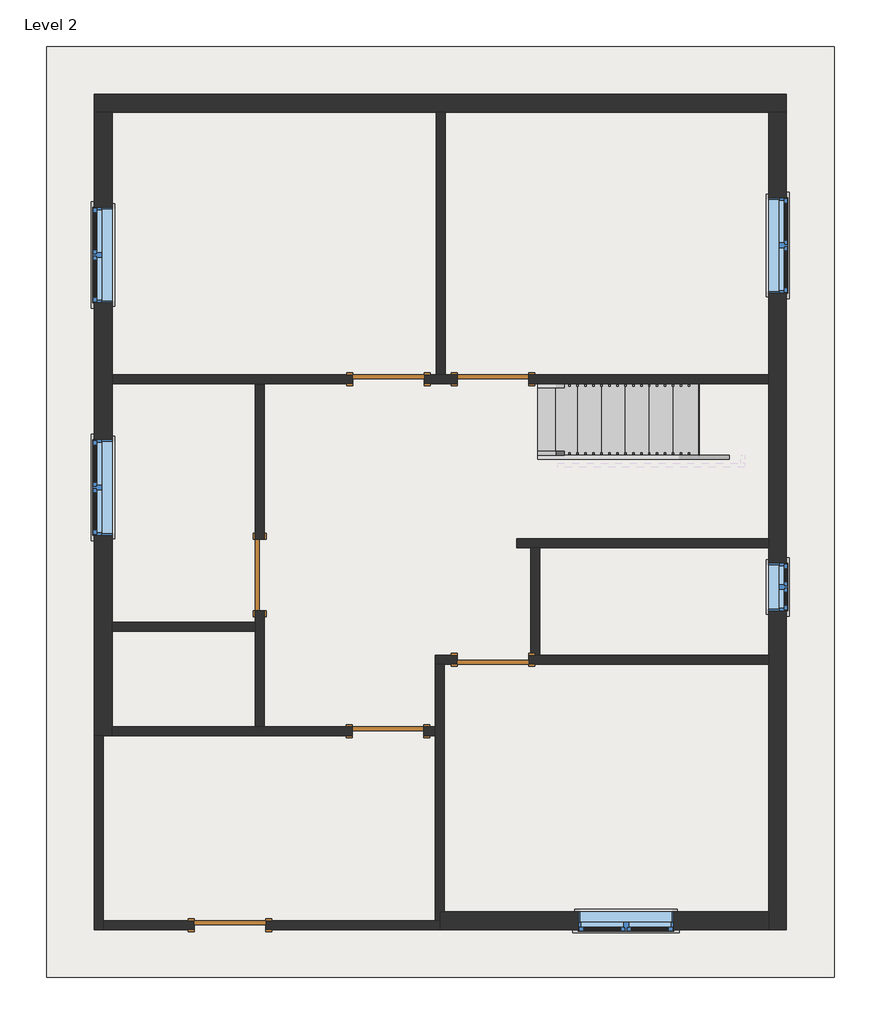
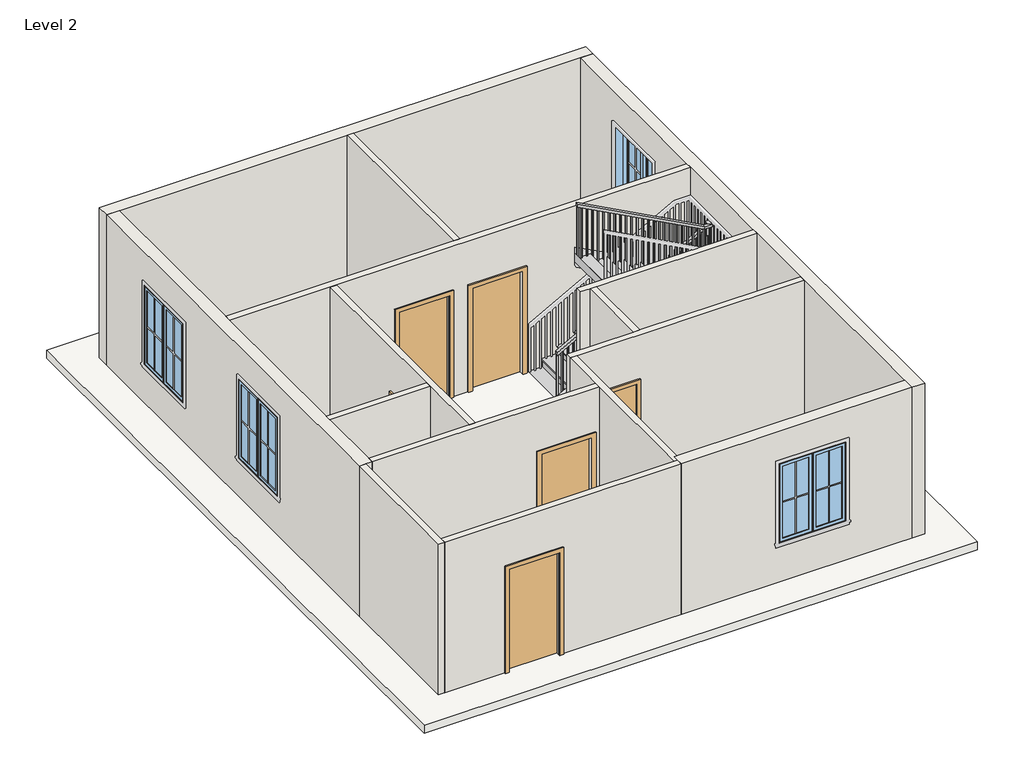
# One storey, part 1 of 2: 15 walls, 6 doors, 5 windows, 1 railing, 1 roof, 1 stair flight.
"""IFC4 building model written with IfcOpenShell, lengths in millimetres."""

from ifc_helpers import new_model, si_unit, frame, origin, place, context, project, spatial, polyline, outline, extrude, faceted_brep, transform, mapped, element, save
from components import door_305aa2a5, door_e5f9f3c4, stair_flight_3d163d7c, window_c417fced, window_8377141f

model = new_model("IFC4")

# Units and contexts
model_context = context("Model", 3, world=origin())
ifc_project = project(units=[si_unit("LENGTHUNIT", "METRE", prefix="MILLI")], contexts=[model_context])

# Site, building, storey
site = spatial("IfcSite", under=ifc_project)
building = spatial("IfcBuilding", under=site)
storey = spatial("IfcBuildingStorey", under=building, Name="Level 2", Elevation=3048.0)

# Doors
placement = place(None, origin())
door_shape = door_305aa2a5(model_context)
element("IfcDoor", 1, ObjectType="Single-Flush : 36\" x 84\"", at=placement, inside=storey, context=model_context, shape_type="MappedRepresentation", body=[
    mapped(door_shape, transform((8001.0, 9251.95, 3048.0), x_axis=(-1.0, 0.0, 0.0), y_axis=(0.0, -1.0, 0.0), z_axis=(0.0, 0.0, 1.0))),
])
element("IfcDoor", 2, ObjectType="Single-Flush : 36\" x 84\"", at=placement, inside=storey, context=model_context, shape_type="MappedRepresentation", body=[
    mapped(door_shape, transform((5022.9818578, 6750.05, 3048.0), x_axis=(0.0, -1.0, 0.0), y_axis=(1.0, 0.0, 0.0), z_axis=(0.0, 0.0, 1.0))),
])
door_2_shape = door_e5f9f3c4(model_context)
element("IfcDoor", 3, ObjectType="Single-Flush : 36\" x 84\"", at=placement, inside=storey, context=model_context, shape_type="MappedRepresentation", body=[
    mapped(door_2_shape, transform((6667.5, 9251.95, 3048.0), x_axis=(1.0, 0.0, 0.0), y_axis=(0.0, 1.0, 0.0), z_axis=(0.0, 0.0, 1.0))),
])
element("IfcDoor", 4, ObjectType="Single-Flush : 36\" x 84\"", at=placement, inside=storey, context=model_context, shape_type="MappedRepresentation", body=[
    mapped(door_2_shape, transform((8001.0, 5670.55, 3048.0), x_axis=(-1.0, 0.0, 0.0), y_axis=(0.0, -1.0, 0.0), z_axis=(0.0, 0.0, 1.0))),
])
element("IfcDoor", 5, ObjectType="Single-Flush : 36\" x 84\"", at=placement, inside=storey, context=model_context, shape_type="MappedRepresentation", body=[
    mapped(door_2_shape, transform((6658.76875, 4756.15, 3048.0), x_axis=(1.0, 0.0, 0.0), y_axis=(0.0, 1.0, 0.0), z_axis=(0.0, 0.0, 1.0))),
])
element("IfcDoor", 6, ObjectType="Single-Flush : 36\" x 84\"", at=placement, inside=storey, context=model_context, shape_type="MappedRepresentation", body=[
    mapped(door_2_shape, transform((4641.85, 2279.65, 3048.0), x_axis=(1.0, 0.0, 0.0), y_axis=(0.0, 1.0, 0.0), z_axis=(0.0, 0.0, 1.0))),
])

# Railing
element("IfcRailing", 7, ObjectType="Handrail - Rectangular", at=placement, inside=storey, context=model_context, shape_type="SolidModel", body=[
    faceted_brep([(8572.5, 8331.2, 4122.8210526), (8572.5, 8331.2, 4064.9285199), (8572.5, 8280.4, 4064.9285199), (8572.5, 8280.4, 4122.8210526), (11137.9, 8331.2, 5524.962753), (11188.7, 8331.2, 5494.8354025), (11188.7, 8280.4, 5494.8354025), (11137.9, 8280.4, 5524.962753), (11137.9, 8331.2, 5566.6105263), (11188.7, 8331.2, 5515.8105263), (11188.7, 8280.4, 5515.8105263), (11137.9, 8280.4, 5566.6105263), (11264.9, 8331.2, 5566.6105263), (11264.9, 8331.2, 5515.8105263), (11214.1, 8280.4, 5515.8105263), (11214.1, 8280.4, 5566.6105263), (11264.9, 8204.2, 5566.6105263), (11264.9, 8153.4, 5515.8105263), (11214.1, 8153.4, 5515.8105263), (11214.1, 8204.2, 5566.6105263), (11264.9, 8204.2, 5767.9901456), (11264.9, 8153.4, 5717.1901456), (11214.1, 8153.4, 5717.1901456), (11214.1, 8204.2, 5767.9901456), (11264.9, 8077.2, 5767.9901456), (11264.9, 8077.2, 5717.1901456), (11214.1, 8128.0, 5717.1901456), (11214.1, 8128.0, 5767.9901456), (11137.9, 8077.2, 5767.9901456), (11125.1122768, 8077.2, 5717.1901456), (11125.1122768, 8128.0, 5717.1901456), (11137.9, 8128.0, 5767.9901456), (8826.5, 8077.2, 7010.4), (8826.5, 8128.0, 7010.4), (8826.5, 8128.0, 6952.7264198), (8826.5, 8077.2, 6952.7264198)], [[[0, 1, 2, 3]], [[1, 0, 4, 5]], [[2, 1, 5, 6]], [[3, 2, 6, 7]], [[0, 3, 7, 4]], [[5, 4, 8, 9]], [[6, 5, 9, 10]], [[7, 6, 10, 11]], [[4, 7, 11, 8]], [[9, 8, 12, 13]], [[10, 9, 13, 14]], [[11, 10, 14, 15]], [[8, 11, 15, 12]], [[13, 12, 16, 17]], [[14, 13, 17, 18]], [[15, 14, 18, 19]], [[12, 15, 19, 16]], [[17, 16, 20, 21]], [[18, 17, 21, 22]], [[19, 18, 22, 23]], [[16, 19, 23, 20]], [[21, 20, 24, 25]], [[22, 21, 25, 26]], [[23, 22, 26, 27]], [[20, 23, 27, 24]], [[25, 24, 28, 29]], [[26, 25, 29, 30]], [[27, 26, 30, 31]], [[24, 27, 31, 28]], [[32, 33, 34, 35]], [[29, 28, 32, 35]], [[30, 29, 35, 34]], [[31, 30, 34, 33]], [[28, 31, 33, 32]]]),
    extrude(outline(polyline([(6906.6480323, 8912.225), (6916.887674, 8893.175), (5935.5789474, 8893.175), (5935.5789474, 8912.225), (6906.6480323, 8912.225)])), frame((0.0, 8093.075, 0.0), z_axis=(0.0, 1.0, 0.0), x_axis=(0.0, 0.0, 1.0)), (0.0, 0.0, 1.0), 19.05),
    extrude(outline(polyline([(6852.0366101, 9013.825), (6862.2762518, 8994.775), (5935.5789474, 8994.775), (5935.5789474, 9013.825), (6852.0366101, 9013.825)])), frame((0.0, 8093.075, 0.0), z_axis=(0.0, 1.0, 0.0), x_axis=(0.0, 0.0, 1.0)), (0.0, 0.0, 1.0), 19.05),
    extrude(outline(polyline([(6797.425188, 9115.425), (6807.6648296, 9096.375), (5775.1578947, 9096.375), (5775.1578947, 9115.425), (6797.425188, 9115.425)])), frame((0.0, 8093.075, 0.0), z_axis=(0.0, 1.0, 0.0), x_axis=(0.0, 0.0, 1.0)), (0.0, 0.0, 1.0), 19.05),
    extrude(outline(polyline([(6742.8137658, 9217.025), (6753.0534074, 9197.975), (5775.1578947, 9197.975), (5775.1578947, 9217.025), (6742.8137658, 9217.025)])), frame((0.0, 8093.075, 0.0), z_axis=(0.0, 1.0, 0.0), x_axis=(0.0, 0.0, 1.0)), (0.0, 0.0, 1.0), 19.05),
    extrude(outline(polyline([(6688.1597952, 9318.625), (6698.5717386, 9299.575), (5775.1578947, 9299.575), (5775.1578947, 9318.625), (6688.1597952, 9318.625)])), frame((0.0, 8093.075, 0.0), z_axis=(0.0, 1.0, 0.0), x_axis=(0.0, 0.0, 1.0)), (0.0, 0.0, 1.0), 19.05),
    extrude(outline(polyline([(6633.5909214, 9420.225), (6643.8305631, 9401.175), (5614.7368421, 9401.175), (5614.7368421, 9420.225), (6633.5909214, 9420.225)])), frame((0.0, 8093.075, 0.0), z_axis=(0.0, 1.0, 0.0), x_axis=(0.0, 0.0, 1.0)), (0.0, 0.0, 1.0), 19.05),
    extrude(outline(polyline([(6578.9794993, 9521.825), (6589.2191409, 9502.775), (5614.7368421, 9502.775), (5614.7368421, 9521.825), (6578.9794993, 9521.825)])), frame((0.0, 8093.075, 0.0), z_axis=(0.0, 1.0, 0.0), x_axis=(0.0, 0.0, 1.0)), (0.0, 0.0, 1.0), 19.05),
    extrude(outline(polyline([(6524.3680771, 9623.425), (6534.6077187, 9604.375), (5614.7368421, 9604.375), (5614.7368421, 9623.425), (6524.3680771, 9623.425)])), frame((0.0, 8093.075, 0.0), z_axis=(0.0, 1.0, 0.0), x_axis=(0.0, 0.0, 1.0)), (0.0, 0.0, 1.0), 19.05),
    extrude(outline(polyline([(6469.7566549, 9725.025), (6479.9962966, 9705.975), (5454.3157895, 9705.975), (5454.3157895, 9725.025), (6469.7566549, 9725.025)])), frame((0.0, 8093.075, 0.0), z_axis=(0.0, 1.0, 0.0), x_axis=(0.0, 0.0, 1.0)), (0.0, 0.0, 1.0), 19.05),
    extrude(outline(polyline([(6415.1452327, 9826.625), (6425.3848744, 9807.575), (5454.3157895, 9807.575), (5454.3157895, 9826.625), (6415.1452327, 9826.625)])), frame((0.0, 8093.075, 0.0), z_axis=(0.0, 1.0, 0.0), x_axis=(0.0, 0.0, 1.0)), (0.0, 0.0, 1.0), 19.05),
    extrude(outline(polyline([(6360.5338106, 9928.225), (6370.7734522, 9909.175), (5454.3157895, 9909.175), (5454.3157895, 9928.225), (6360.5338106, 9928.225)])), frame((0.0, 8093.075, 0.0), z_axis=(0.0, 1.0, 0.0), x_axis=(0.0, 0.0, 1.0)), (0.0, 0.0, 1.0), 19.05),
    extrude(outline(polyline([(6305.9223884, 10029.825), (6316.1620301, 10010.775), (5293.8947368, 10010.775), (5293.8947368, 10029.825), (6305.9223884, 10029.825)])), frame((0.0, 8093.075, 0.0), z_axis=(0.0, 1.0, 0.0), x_axis=(0.0, 0.0, 1.0)), (0.0, 0.0, 1.0), 19.05),
    extrude(outline(polyline([(6251.3109662, 10131.425), (6261.5506079, 10112.375), (5293.8947368, 10112.375), (5293.8947368, 10131.425), (6251.3109662, 10131.425)])), frame((0.0, 8093.075, 0.0), z_axis=(0.0, 1.0, 0.0), x_axis=(0.0, 0.0, 1.0)), (0.0, 0.0, 1.0), 19.05),
    extrude(outline(polyline([(6196.6995441, 10233.025), (6206.9391857, 10213.975), (5293.8947368, 10213.975), (5293.8947368, 10233.025), (6196.6995441, 10233.025)])), frame((0.0, 8093.075, 0.0), z_axis=(0.0, 1.0, 0.0), x_axis=(0.0, 0.0, 1.0)), (0.0, 0.0, 1.0), 19.05),
    extrude(outline(polyline([(6142.0881219, 10334.625), (6152.3277635, 10315.575), (5133.4736842, 10315.575), (5133.4736842, 10334.625), (6142.0881219, 10334.625)])), frame((0.0, 8093.075, 0.0), z_axis=(0.0, 1.0, 0.0), x_axis=(0.0, 0.0, 1.0)), (0.0, 0.0, 1.0), 19.05),
    extrude(outline(polyline([(6087.4766997, 10436.225), (6097.7163414, 10417.175), (5133.4736842, 10417.175), (5133.4736842, 10436.225), (6087.4766997, 10436.225)])), frame((0.0, 8093.075, 0.0), z_axis=(0.0, 1.0, 0.0), x_axis=(0.0, 0.0, 1.0)), (0.0, 0.0, 1.0), 19.05),
    extrude(outline(polyline([(6032.8652775, 10537.825), (6043.1049192, 10518.775), (5133.4736842, 10518.775), (5133.4736842, 10537.825), (6032.8652775, 10537.825)])), frame((0.0, 8093.075, 0.0), z_axis=(0.0, 1.0, 0.0), x_axis=(0.0, 0.0, 1.0)), (0.0, 0.0, 1.0), 19.05),
    extrude(outline(polyline([(5978.2538554, 10639.425), (5988.493497, 10620.375), (4973.0526316, 10620.375), (4973.0526316, 10639.425), (5978.2538554, 10639.425)])), frame((0.0, 8093.075, 0.0), z_axis=(0.0, 1.0, 0.0), x_axis=(0.0, 0.0, 1.0)), (0.0, 0.0, 1.0), 19.05),
    extrude(outline(polyline([(5923.6424332, 10741.025), (5933.8820749, 10721.975), (4973.0526316, 10721.975), (4973.0526316, 10741.025), (5923.6424332, 10741.025)])), frame((0.0, 8093.075, 0.0), z_axis=(0.0, 1.0, 0.0), x_axis=(0.0, 0.0, 1.0)), (0.0, 0.0, 1.0), 19.05),
    extrude(outline(polyline([(5869.031011, 10842.625), (5879.2706527, 10823.575), (4973.0526316, 10823.575), (4973.0526316, 10842.625), (5869.031011, 10842.625)])), frame((0.0, 8093.075, 0.0), z_axis=(0.0, 1.0, 0.0), x_axis=(0.0, 0.0, 1.0)), (0.0, 0.0, 1.0), 19.05),
    extrude(outline(polyline([(5814.4195889, 10944.225), (5824.6592305, 10925.175), (4812.6315789, 10925.175), (4812.6315789, 10944.225), (5814.4195889, 10944.225)])), frame((0.0, 8093.075, 0.0), z_axis=(0.0, 1.0, 0.0), x_axis=(0.0, 0.0, 1.0)), (0.0, 0.0, 1.0), 19.05),
    extrude(outline(polyline([(5759.8081667, 11045.825), (5770.0478083, 11026.775), (4812.6315789, 11026.775), (4812.6315789, 11045.825), (5759.8081667, 11045.825)])), frame((0.0, 8093.075, 0.0), z_axis=(0.0, 1.0, 0.0), x_axis=(0.0, 0.0, 1.0)), (0.0, 0.0, 1.0), 19.05),
    extrude(outline(polyline([(5705.1967445, 11147.425), (5715.4363862, 11128.375), (4812.6315789, 11128.375), (4812.6315789, 11147.425), (5705.1967445, 11147.425)])), frame((0.0, 8093.075, 0.0), z_axis=(0.0, 1.0, 0.0), x_axis=(0.0, 0.0, 1.0)), (0.0, 0.0, 1.0), 19.05),
    extrude(outline(polyline([(11229.975, 8213.725), (11249.025, 8213.725), (11249.025, 8194.675), (11229.975, 8194.675), (11229.975, 8213.725)])), frame((0.0, 0.0, 4652.2105263), z_axis=(0.0, 0.0, 1.0), x_axis=(1.0, 0.0, 0.0)), (0.0, 0.0, 1.0), 863.6),
    extrude(outline(polyline([(11204.575, 8296.275), (11204.575, 8315.325), (11223.625, 8315.325), (11223.625, 8296.275), (11204.575, 8296.275)])), frame((0.0, 0.0, 4652.2105263), z_axis=(0.0, 0.0, 1.0), x_axis=(1.0, 0.0, 0.0)), (0.0, 0.0, 1.0), 863.6),
    extrude(outline(polyline([(5458.3936009, 11122.025), (5447.9816576, 11102.975), (4491.7894737, 11102.975), (4491.7894737, 11122.025), (5458.3936009, 11122.025)])), frame((0.0, 8296.275, 0.0), z_axis=(0.0, 1.0, 0.0), x_axis=(0.0, 0.0, 1.0)), (0.0, 0.0, 1.0), 19.05),
    extrude(outline(polyline([(5402.8632365, 11020.425), (5392.4512932, 11001.375), (4491.7894737, 11001.375), (4491.7894737, 11020.425), (5402.8632365, 11020.425)])), frame((0.0, 8296.275, 0.0), z_axis=(0.0, 1.0, 0.0), x_axis=(0.0, 0.0, 1.0)), (0.0, 0.0, 1.0), 19.05),
    extrude(outline(polyline([(5347.3328722, 10918.825), (5336.9209288, 10899.775), (4491.7894737, 10899.775), (4491.7894737, 10918.825), (5347.3328722, 10918.825)])), frame((0.0, 8296.275, 0.0), z_axis=(0.0, 1.0, 0.0), x_axis=(0.0, 0.0, 1.0)), (0.0, 0.0, 1.0), 19.05),
    extrude(outline(polyline([(5291.8025078, 10817.225), (5281.3905645, 10798.175), (4331.3684211, 10798.175), (4331.3684211, 10817.225), (5291.8025078, 10817.225)])), frame((0.0, 8296.275, 0.0), z_axis=(0.0, 1.0, 0.0), x_axis=(0.0, 0.0, 1.0)), (0.0, 0.0, 1.0), 19.05),
    extrude(outline(polyline([(5236.2721434, 10715.625), (5225.8602001, 10696.575), (4331.3684211, 10696.575), (4331.3684211, 10715.625), (5236.2721434, 10715.625)])), frame((0.0, 8296.275, 0.0), z_axis=(0.0, 1.0, 0.0), x_axis=(0.0, 0.0, 1.0)), (0.0, 0.0, 1.0), 19.05),
    extrude(outline(polyline([(5180.741779, 10614.025), (5170.3298357, 10594.975), (4331.3684211, 10594.975), (4331.3684211, 10614.025), (5180.741779, 10614.025)])), frame((0.0, 8296.275, 0.0), z_axis=(0.0, 1.0, 0.0), x_axis=(0.0, 0.0, 1.0)), (0.0, 0.0, 1.0), 19.05),
    extrude(outline(polyline([(5125.2114147, 10512.425), (5114.7994714, 10493.375), (4170.9473684, 10493.375), (4170.9473684, 10512.425), (5125.2114147, 10512.425)])), frame((0.0, 8296.275, 0.0), z_axis=(0.0, 1.0, 0.0), x_axis=(0.0, 0.0, 1.0)), (0.0, 0.0, 1.0), 19.05),
    extrude(outline(polyline([(5069.6810503, 10410.825), (5059.269107, 10391.775), (4170.9473684, 10391.775), (4170.9473684, 10410.825), (5069.6810503, 10410.825)])), frame((0.0, 8296.275, 0.0), z_axis=(0.0, 1.0, 0.0), x_axis=(0.0, 0.0, 1.0)), (0.0, 0.0, 1.0), 19.05),
    extrude(outline(polyline([(5014.1506859, 10309.225), (5003.7387426, 10290.175), (4170.9473684, 10290.175), (4170.9473684, 10309.225), (5014.1506859, 10309.225)])), frame((0.0, 8296.275, 0.0), z_axis=(0.0, 1.0, 0.0), x_axis=(0.0, 0.0, 1.0)), (0.0, 0.0, 1.0), 19.05),
    extrude(outline(polyline([(4958.6203216, 10207.625), (4948.2083782, 10188.575), (4010.5263158, 10188.575), (4010.5263158, 10207.625), (4958.6203216, 10207.625)])), frame((0.0, 8296.275, 0.0), z_axis=(0.0, 1.0, 0.0), x_axis=(0.0, 0.0, 1.0)), (0.0, 0.0, 1.0), 19.05),
    extrude(outline(polyline([(4903.0899572, 10106.025), (4892.6780139, 10086.975), (4010.5263158, 10086.975), (4010.5263158, 10106.025), (4903.0899572, 10106.025)])), frame((0.0, 8296.275, 0.0), z_axis=(0.0, 1.0, 0.0), x_axis=(0.0, 0.0, 1.0)), (0.0, 0.0, 1.0), 19.05),
    extrude(outline(polyline([(4847.5595928, 10004.425), (4837.1476495, 9985.375), (4010.5263158, 9985.375), (4010.5263158, 10004.425), (4847.5595928, 10004.425)])), frame((0.0, 8296.275, 0.0), z_axis=(0.0, 1.0, 0.0), x_axis=(0.0, 0.0, 1.0)), (0.0, 0.0, 1.0), 19.05),
    extrude(outline(polyline([(4792.0292284, 9902.825), (4781.6172851, 9883.775), (3850.1052632, 9883.775), (3850.1052632, 9902.825), (4792.0292284, 9902.825)])), frame((0.0, 8296.275, 0.0), z_axis=(0.0, 1.0, 0.0), x_axis=(0.0, 0.0, 1.0)), (0.0, 0.0, 1.0), 19.05),
    extrude(outline(polyline([(4736.4988641, 9801.225), (4726.0869207, 9782.175), (3850.1052632, 9782.175), (3850.1052632, 9801.225), (4736.4988641, 9801.225)])), frame((0.0, 8296.275, 0.0), z_axis=(0.0, 1.0, 0.0), x_axis=(0.0, 0.0, 1.0)), (0.0, 0.0, 1.0), 19.05),
    extrude(outline(polyline([(4680.9684997, 9699.625), (4670.5565564, 9680.575), (3850.1052632, 9680.575), (3850.1052632, 9699.625), (4680.9684997, 9699.625)])), frame((0.0, 8296.275, 0.0), z_axis=(0.0, 1.0, 0.0), x_axis=(0.0, 0.0, 1.0)), (0.0, 0.0, 1.0), 19.05),
    extrude(outline(polyline([(4625.4381353, 9598.025), (4615.026192, 9578.975), (3689.6842105, 9578.975), (3689.6842105, 9598.025), (4625.4381353, 9598.025)])), frame((0.0, 8296.275, 0.0), z_axis=(0.0, 1.0, 0.0), x_axis=(0.0, 0.0, 1.0)), (0.0, 0.0, 1.0), 19.05),
    extrude(outline(polyline([(4569.9077709, 9496.425), (4559.4958276, 9477.375), (3689.6842105, 9477.375), (3689.6842105, 9496.425), (4569.9077709, 9496.425)])), frame((0.0, 8296.275, 0.0), z_axis=(0.0, 1.0, 0.0), x_axis=(0.0, 0.0, 1.0)), (0.0, 0.0, 1.0), 19.05),
    extrude(outline(polyline([(4514.3774066, 9394.825), (4503.9654633, 9375.775), (3689.6842105, 9375.775), (3689.6842105, 9394.825), (4514.3774066, 9394.825)])), frame((0.0, 8296.275, 0.0), z_axis=(0.0, 1.0, 0.0), x_axis=(0.0, 0.0, 1.0)), (0.0, 0.0, 1.0), 19.05),
    extrude(outline(polyline([(4458.8470422, 9293.225), (4448.4350989, 9274.175), (3529.2631579, 9274.175), (3529.2631579, 9293.225), (4458.8470422, 9293.225)])), frame((0.0, 8296.275, 0.0), z_axis=(0.0, 1.0, 0.0), x_axis=(0.0, 0.0, 1.0)), (0.0, 0.0, 1.0), 19.05),
    extrude(outline(polyline([(4403.3166778, 9191.625), (4392.9047345, 9172.575), (3529.2631579, 9172.575), (3529.2631579, 9191.625), (4403.3166778, 9191.625)])), frame((0.0, 8296.275, 0.0), z_axis=(0.0, 1.0, 0.0), x_axis=(0.0, 0.0, 1.0)), (0.0, 0.0, 1.0), 19.05),
    extrude(outline(polyline([(4347.7863135, 9090.025), (4337.3743701, 9070.975), (3529.2631579, 9070.975), (3529.2631579, 9090.025), (4347.7863135, 9090.025)])), frame((0.0, 8296.275, 0.0), z_axis=(0.0, 1.0, 0.0), x_axis=(0.0, 0.0, 1.0)), (0.0, 0.0, 1.0), 19.05),
    extrude(outline(polyline([(4292.2559491, 8988.425), (4281.8440058, 8969.375), (3368.8421053, 8969.375), (3368.8421053, 8988.425), (4292.2559491, 8988.425)])), frame((0.0, 8296.275, 0.0), z_axis=(0.0, 1.0, 0.0), x_axis=(0.0, 0.0, 1.0)), (0.0, 0.0, 1.0), 19.05),
    extrude(outline(polyline([(4236.7255847, 8886.825), (4226.3136414, 8867.775), (3368.8421053, 8867.775), (3368.8421053, 8886.825), (4236.7255847, 8886.825)])), frame((0.0, 8296.275, 0.0), z_axis=(0.0, 1.0, 0.0), x_axis=(0.0, 0.0, 1.0)), (0.0, 0.0, 1.0), 19.05),
    extrude(outline(polyline([(4181.1952203, 8785.225), (4170.783277, 8766.175), (3208.4210526, 8766.175), (3208.4210526, 8785.225), (4181.1952203, 8785.225)])), frame((0.0, 8296.275, 0.0), z_axis=(0.0, 1.0, 0.0), x_axis=(0.0, 0.0, 1.0)), (0.0, 0.0, 1.0), 19.05),
    extrude(outline(polyline([(4125.664856, 8683.625), (4115.2529126, 8664.575), (3208.4210526, 8664.575), (3208.4210526, 8683.625), (4125.664856, 8683.625)])), frame((0.0, 8296.275, 0.0), z_axis=(0.0, 1.0, 0.0), x_axis=(0.0, 0.0, 1.0)), (0.0, 0.0, 1.0), 19.05),
    extrude(outline(polyline([(11229.975, 8112.125), (11249.025, 8112.125), (11249.025, 8093.075), (11229.975, 8093.075), (11229.975, 8112.125)])), frame((0.0, 0.0, 4652.2105263), z_axis=(0.0, 0.0, 1.0), x_axis=(1.0, 0.0, 0.0)), (0.0, 0.0, 1.0), 1064.9796193),
    extrude(outline(polyline([(11229.975, 8296.275), (11229.975, 8315.325), (11249.025, 8315.325), (11249.025, 8296.275), (11229.975, 8296.275)])), frame((0.0, 0.0, 4652.2105263), z_axis=(0.0, 0.0, 1.0), x_axis=(1.0, 0.0, 0.0)), (0.0, 0.0, 1.0), 863.6),
    extrude(outline(polyline([(6942.4867781, 8845.55), (6952.7264198, 8826.5), (5935.5789474, 8826.5), (5935.5789474, 8845.55), (6942.4867781, 8845.55)])), frame((0.0, 8093.075, 0.0), z_axis=(0.0, 1.0, 0.0), x_axis=(0.0, 0.0, 1.0)), (0.0, 0.0, 1.0), 19.05),
    extrude(outline(polyline([(4075.3404633, 8591.55), (4064.9285199, 8572.5), (3208.4210526, 8572.5), (3208.4210526, 8591.55), (4075.3404633, 8591.55)])), frame((0.0, 8296.275, 0.0), z_axis=(0.0, 1.0, 0.0), x_axis=(0.0, 0.0, 1.0)), (0.0, 0.0, 1.0), 19.05),
])

# Roof
element("IfcRoof", 8, ObjectType="Generic - 12\"", at=placement, inside=storey, context=model_context, shape_type="SweptSolid", body=[
    extrude(outline(polyline([(2298.7, 13500.1), (12357.1, 13500.1), (12357.1, 1612.9), (2298.7, 1612.9), (2298.7, 13500.1)])), frame((0.0, 0.0, 3048.0), z_axis=(0.0, 0.0, 1.0), x_axis=(1.0, 0.0, 0.0)), (0.0, 0.0, 1.0), 152.4),
])

# Stair flight
stair_flight_shape = stair_flight_3d163d7c(model_context)
element("IfcStairFlight", 9, ObjectType="2\" Tread 1\" Nosing 1/4\" Riser", at=placement, inside=storey, context=model_context, shape_type="MappedRepresentation", body=[
    mapped(stair_flight_shape, transform((0.0, 0.0, 0.0), x_axis=(1.0, 0.0, 0.0), y_axis=(0.0, 1.0, 0.0), z_axis=(0.0, 0.0, 1.0))),
])

# Walls
element("IfcWall", 10, ObjectType="Generic - 5\"", at=placement, inside=storey, context=model_context, shape_type="Brep", body=[
    faceted_brep([(7115.96875, 4699.0, 5181.6), (7115.96875, 4699.0, 3048.0), (7264.4, 4699.0, 3048.0), (7264.4, 4699.0, 6096.0), (3136.9, 4699.0, 6096.0), (3136.9, 4699.0, 3048.0), (6201.56875, 4699.0, 3048.0), (6201.56875, 4699.0, 5181.6), (7264.4, 4813.3, 3048.0), (7115.96875, 4813.3, 3048.0), (7115.96875, 4813.3, 5181.6), (6201.56875, 4813.3, 5181.6), (6201.56875, 4813.3, 3048.0), (5080.1318578, 4813.3, 3048.0), (4965.8318578, 4813.3, 3048.0), (3136.9, 4813.3, 3048.0), (3136.9, 4813.3, 6096.0), (4965.8318578, 4813.3, 6096.0), (5080.1318578, 4813.3, 6096.0), (7264.4, 4813.3, 6096.0)], [[[0, 1, 2, 3, 4, 5, 6, 7]], [[8, 9, 10, 11, 12, 13, 14, 15, 16, 17, 18, 19]], [[6, 5, 15, 14, 13, 12]], [[2, 1, 9, 8]], [[4, 3, 19, 18, 17, 16]], [[5, 4, 16, 15]], [[3, 2, 8, 19]], [[10, 9, 1, 0]], [[11, 10, 0, 7]], [[12, 11, 7, 6]]]),
])
element("IfcWall", 11, ObjectType="Generic - 5\"", at=placement, inside=storey, context=model_context, shape_type="SweptSolid", body=[
    extrude(outline(polyline([(4965.8318578, 6032.5), (3136.9, 6032.5), (3136.9, 6146.8), (4965.8318578, 6146.8), (4965.8318578, 6032.5)])), frame((0.0, 0.0, 3048.0), z_axis=(0.0, 0.0, 1.0), x_axis=(1.0, 0.0, 0.0)), (0.0, 0.0, 1.0), 3048.0),
])
element("IfcWall", 12, ObjectType="Generic - 5\"", at=placement, inside=storey, context=model_context, shape_type="Brep", body=[
    faceted_brep([(5080.1318578, 4813.3, 3048.0), (5080.1318578, 6292.85, 3048.0), (5080.1318578, 6292.85, 5181.6), (5080.1318578, 7207.25, 5181.6), (5080.1318578, 7207.25, 3048.0), (5080.1318578, 9182.1, 3048.0), (5080.1318578, 9182.1, 6096.0), (5080.1318578, 4813.3, 6096.0), (4965.8318578, 6292.85, 5181.6), (4965.8318578, 6292.85, 3048.0), (4965.8318578, 6146.8, 3048.0), (4965.8318578, 6032.5, 3048.0), (4965.8318578, 4813.3, 3048.0), (4965.8318578, 4813.3, 6096.0), (4965.8318578, 6032.5, 6096.0), (4965.8318578, 6146.8, 6096.0), (4965.8318578, 9182.1, 6096.0), (4965.8318578, 9182.1, 3048.0), (4965.8318578, 7207.25, 3048.0), (4965.8318578, 7207.25, 5181.6)], [[[0, 1, 2, 3, 4, 5, 6, 7]], [[8, 9, 10, 11, 12, 13, 14, 15, 16, 17, 18, 19]], [[18, 17, 5, 4]], [[12, 11, 10, 9, 1, 0]], [[6, 5, 17, 16]], [[7, 6, 16, 15, 14, 13]], [[0, 7, 13, 12]], [[2, 1, 9, 8]], [[3, 2, 8, 19]], [[4, 3, 19, 18]]]),
])
element("IfcWall", 13, ObjectType="Generic - 5\"", at=placement, inside=storey, context=model_context, shape_type="Brep", body=[
    faceted_brep([(7124.7, 9194.8, 5181.6), (7124.7, 9194.8, 3048.0), (7543.8, 9194.8, 3048.0), (7543.8, 9194.8, 5181.6), (8458.2, 9194.8, 5181.6), (8458.2, 9194.8, 3048.0), (11518.9, 9194.8, 3048.0), (11518.9, 9194.8, 6096.0), (3136.9, 9194.8, 6096.0), (3136.9, 9194.8, 3048.0), (6210.3, 9194.8, 3048.0), (6210.3, 9194.8, 5181.6), (7543.8, 9309.1, 3048.0), (7391.4, 9309.1, 3048.0), (7277.1, 9309.1, 3048.0), (7124.7, 9309.1, 3048.0), (7124.7, 9309.1, 5181.6), (6210.3, 9309.1, 5181.6), (6210.3, 9309.1, 3048.0), (3136.9, 9309.1, 3048.0), (3136.9, 9309.1, 6096.0), (7277.1, 9309.1, 6096.0), (7391.4, 9309.1, 6096.0), (11518.9, 9309.1, 6096.0), (11518.9, 9309.1, 3048.0), (8458.2, 9309.1, 3048.0), (8458.2, 9309.1, 5181.6), (7543.8, 9309.1, 5181.6)], [[[0, 1, 2, 3, 4, 5, 6, 7, 8, 9, 10, 11]], [[12, 13, 14, 15, 16, 17, 18, 19, 20, 21, 22, 23, 24, 25, 26, 27]], [[25, 24, 6, 5]], [[10, 9, 19, 18]], [[2, 1, 15, 14, 13, 12]], [[8, 7, 23, 22, 21, 20]], [[7, 6, 24, 23]], [[9, 8, 20, 19]], [[3, 2, 12, 27]], [[4, 3, 27, 26]], [[5, 4, 26, 25]], [[16, 15, 1, 0]], [[17, 16, 0, 11]], [[18, 17, 11, 10]]]),
])
element("IfcWall", 14, ObjectType="Generic - 5\"", at=placement, inside=storey, context=model_context, shape_type="SweptSolid", body=[
    extrude(outline(polyline([(7277.1, 9309.1), (7277.1, 12661.9), (7391.4, 12661.9), (7391.4, 9309.1), (7277.1, 9309.1)])), frame((0.0, 0.0, 3048.0), z_axis=(0.0, 0.0, 1.0), x_axis=(1.0, 0.0, 0.0)), (0.0, 0.0, 1.0), 3048.0),
])
element("IfcWall", 15, ObjectType="Generic - 5\"", at=placement, inside=storey, context=model_context, shape_type="Brep", body=[
    faceted_brep([(2908.3, 4699.0, 3048.0), (2908.3, 2222.5, 3048.0), (2908.3, 2222.5, 6096.0), (2908.3, 4699.0, 6096.0), (3022.6, 4699.0, 3048.0), (3022.6, 4699.0, 6096.0), (3022.6, 2336.8, 6096.0), (3022.6, 2222.5, 6096.0), (3022.6, 2222.5, 3048.0), (3022.6, 2336.8, 3048.0)], [[[0, 1, 2, 3]], [[4, 5, 6, 7, 8, 9]], [[1, 0, 4, 9, 8]], [[3, 2, 7, 6, 5]], [[0, 3, 5, 4]], [[2, 1, 8, 7]]]),
])
element("IfcWall", 16, ObjectType="Generic - 5\"", at=placement, inside=storey, context=model_context, shape_type="Brep", body=[
    faceted_brep([(5099.05, 2222.5, 5181.6), (5099.05, 2222.5, 3048.0), (7321.55, 2222.5, 3048.0), (7321.55, 2222.5, 6096.0), (3022.6, 2222.5, 6096.0), (3022.6, 2222.5, 3048.0), (4184.65, 2222.5, 3048.0), (4184.65, 2222.5, 5181.6), (7321.55, 2336.8, 3048.0), (7264.4, 2336.8, 3048.0), (5099.05, 2336.8, 3048.0), (5099.05, 2336.8, 5181.6), (4184.65, 2336.8, 5181.6), (4184.65, 2336.8, 3048.0), (3022.6, 2336.8, 3048.0), (3022.6, 2336.8, 6096.0), (7264.4, 2336.8, 6096.0), (7321.55, 2336.8, 6096.0)], [[[0, 1, 2, 3, 4, 5, 6, 7]], [[8, 9, 10, 11, 12, 13, 14, 15, 16, 17]], [[6, 5, 14, 13]], [[2, 1, 10, 9, 8]], [[3, 2, 8, 17]], [[4, 3, 17, 16, 15]], [[5, 4, 15, 14]], [[11, 10, 1, 0]], [[12, 11, 0, 7]], [[13, 12, 7, 6]]]),
])
element("IfcWall", 17, ObjectType="Generic - 5\"", at=placement, inside=storey, context=model_context, shape_type="Brep", body=[
    faceted_brep([(11518.9, 7213.6, 3048.0), (8305.8, 7213.6, 3048.0), (8305.8, 7213.6, 6096.0), (11518.9, 7213.6, 6096.0), (11518.9, 7099.3, 3048.0), (11518.9, 7099.3, 6096.0), (8597.9, 7099.3, 6096.0), (8483.6, 7099.3, 6096.0), (8305.8, 7099.3, 6096.0), (8305.8, 7099.3, 3048.0), (8483.6, 7099.3, 3048.0), (8597.9, 7099.3, 3048.0)], [[[0, 1, 2, 3]], [[4, 5, 6, 7, 8, 9, 10, 11]], [[1, 0, 4, 11, 10, 9]], [[2, 1, 9, 8]], [[3, 2, 8, 7, 6, 5]], [[0, 3, 5, 4]]]),
])
element("IfcWall", 18, ObjectType="Generic - 5\"", at=placement, inside=storey, context=model_context, shape_type="SweptSolid", body=[
    extrude(outline(polyline([(8483.6, 5727.7), (8483.6, 7099.3), (8597.9, 7099.3), (8597.9, 5727.7), (8483.6, 5727.7)])), frame((0.0, 0.0, 3048.0), z_axis=(0.0, 0.0, 1.0), x_axis=(1.0, 0.0, 0.0)), (0.0, 0.0, 1.0), 3048.0),
])
element("IfcWall", 19, ObjectType="Generic - 5\"", at=placement, inside=storey, context=model_context, shape_type="Brep", body=[
    faceted_brep([(7543.8, 5727.7, 5181.6), (7543.8, 5727.7, 3048.0), (7264.4, 5727.7, 3048.0), (7264.4, 5727.7, 6096.0), (8483.6, 5727.7, 6096.0), (8597.9, 5727.7, 6096.0), (11518.9, 5727.7, 6096.0), (11518.9, 5727.7, 3048.0), (8597.9, 5727.7, 3048.0), (8483.6, 5727.7, 3048.0), (8458.2, 5727.7, 3048.0), (8458.2, 5727.7, 5181.6), (7264.4, 5613.4, 3048.0), (7378.7, 5613.4, 3048.0), (7543.8, 5613.4, 3048.0), (7543.8, 5613.4, 5181.6), (8458.2, 5613.4, 5181.6), (8458.2, 5613.4, 3048.0), (11518.9, 5613.4, 3048.0), (11518.9, 5613.4, 6096.0), (7378.7, 5613.4, 6096.0), (7264.4, 5613.4, 6096.0)], [[[0, 1, 2, 3, 4, 5, 6, 7, 8, 9, 10, 11]], [[12, 13, 14, 15, 16, 17, 18, 19, 20, 21]], [[2, 1, 14, 13, 12]], [[10, 9, 8, 7, 18, 17]], [[6, 5, 4, 3, 21, 20, 19]], [[7, 6, 19, 18]], [[3, 2, 12, 21]], [[15, 14, 1, 0]], [[16, 15, 0, 11]], [[17, 16, 11, 10]]]),
])
element("IfcWall", 20, ObjectType="Generic - 5\"", at=placement, inside=storey, context=model_context, shape_type="Brep", body=[
    faceted_brep([(7264.4, 5613.4, 3048.0), (7264.4, 4813.3, 3048.0), (7264.4, 4699.0, 3048.0), (7264.4, 2336.8, 3048.0), (7264.4, 2336.8, 6096.0), (7264.4, 4699.0, 6096.0), (7264.4, 4813.3, 6096.0), (7264.4, 5613.4, 6096.0), (7378.7, 5613.4, 3048.0), (7378.7, 5613.4, 6096.0), (7378.7, 2451.1, 6096.0), (7378.7, 2451.1, 3048.0), (7321.55, 2451.1, 3048.0), (7321.55, 2336.8, 3048.0), (7321.55, 2336.8, 6096.0), (7321.55, 2451.1, 6096.0)], [[[0, 1, 2, 3, 4, 5, 6, 7]], [[8, 9, 10, 11]], [[3, 2, 1, 0, 8, 11, 12, 13]], [[7, 6, 5, 4, 14, 15, 10, 9]], [[0, 7, 9, 8]], [[4, 3, 13, 14]], [[13, 12, 15, 14]], [[12, 11, 10, 15]]]),
])
element("IfcWall", 21, ObjectType="Generic - 8\"", at=placement, inside=storey, context=model_context, shape_type="Brep", body=[
    faceted_brep([(2908.3, 12661.9, 3048.0), (3136.9, 12661.9, 3048.0), (7277.1, 12661.9, 3048.0), (7391.4, 12661.9, 3048.0), (11518.9, 12661.9, 3048.0), (11747.5, 12661.9, 3048.0), (11747.5, 12661.9, 6096.0), (11518.9, 12661.9, 6096.0), (7391.4, 12661.9, 6096.0), (7277.1, 12661.9, 6096.0), (3136.9, 12661.9, 6096.0), (2908.3, 12661.9, 6096.0), (2908.3, 12890.5, 3048.0), (2908.3, 12890.5, 6096.0), (11747.5, 12890.5, 6096.0), (11747.5, 12890.5, 3048.0)], [[[0, 1, 2, 3, 4, 5, 6, 7, 8, 9, 10, 11]], [[12, 13, 14, 15]], [[5, 4, 3, 2, 1, 0, 12, 15]], [[11, 10, 9, 8, 7, 6, 14, 13]], [[6, 5, 15, 14]], [[0, 11, 13, 12]]]),
])
element("IfcWall", 22, ObjectType="Generic - 8\"", at=placement, inside=storey, context=model_context, shape_type="Brep", body=[
    faceted_brep([(11518.9, 12661.9, 3048.0), (11518.9, 9309.1, 3048.0), (11518.9, 9194.8, 3048.0), (11518.9, 7213.6, 3048.0), (11518.9, 7099.3, 3048.0), (11518.9, 5727.7, 3048.0), (11518.9, 5613.4, 3048.0), (11518.9, 2451.1, 3048.0), (11518.9, 2222.5, 3048.0), (11518.9, 2222.5, 6096.0), (11518.9, 2451.1, 6096.0), (11518.9, 5613.4, 6096.0), (11518.9, 5727.7, 6096.0), (11518.9, 7099.3, 6096.0), (11518.9, 7213.6, 6096.0), (11518.9, 9194.8, 6096.0), (11518.9, 9309.1, 6096.0), (11518.9, 12661.9, 6096.0), (11518.9, 10352.0875, 5486.4), (11518.9, 10352.0875, 3962.4), (11518.9, 11571.2875, 3962.4), (11518.9, 11571.2875, 5486.4), (11518.9, 6292.85, 4876.8), (11518.9, 6292.85, 3962.4), (11518.9, 6902.45, 3962.4), (11518.9, 6902.45, 4876.8), (11747.5, 12661.9, 3048.0), (11747.5, 12661.9, 6096.0), (11747.5, 2222.5, 6096.0), (11747.5, 2222.5, 3048.0), (11747.5, 10352.0875, 5486.4), (11747.5, 11571.2875, 5486.4), (11747.5, 11571.2875, 3962.4), (11747.5, 10352.0875, 3962.4), (11747.5, 6292.85, 4876.8), (11747.5, 6902.45, 4876.8), (11747.5, 6902.45, 3962.4), (11747.5, 6292.85, 3962.4)], [[[0, 1, 2, 3, 4, 5, 6, 7, 8, 9, 10, 11, 12, 13, 14, 15, 16, 17], [18, 19, 20, 21], [22, 23, 24, 25]], [[26, 27, 28, 29], [30, 31, 32, 33], [34, 35, 36, 37]], [[8, 7, 6, 5, 4, 3, 2, 1, 0, 26, 29]], [[17, 16, 15, 14, 13, 12, 11, 10, 9, 28, 27]], [[0, 17, 27, 26]], [[9, 8, 29, 28]], [[19, 18, 30, 33]], [[20, 19, 33, 32]], [[21, 20, 32, 31]], [[18, 21, 31, 30]], [[23, 22, 34, 37]], [[24, 23, 37, 36]], [[25, 24, 36, 35]], [[22, 25, 35, 34]]]),
])
element("IfcWall", 23, ObjectType="Generic - 8\"", at=placement, inside=storey, context=model_context, shape_type="Brep", body=[
    faceted_brep([(2908.3, 12661.9, 3048.0), (2908.3, 4699.0, 3048.0), (2908.3, 4699.0, 6096.0), (2908.3, 12661.9, 6096.0), (2908.3, 8480.425, 5486.4), (2908.3, 7261.225, 5486.4), (2908.3, 7261.225, 3962.4), (2908.3, 8480.425, 3962.4), (2908.3, 11449.05, 5486.4), (2908.3, 10229.85, 5486.4), (2908.3, 10229.85, 3962.4), (2908.3, 11449.05, 3962.4), (3136.9, 12661.9, 3048.0), (3136.9, 12661.9, 6096.0), (3136.9, 9309.1, 6096.0), (3136.9, 9194.8, 6096.0), (3136.9, 6146.8, 6096.0), (3136.9, 6032.5, 6096.0), (3136.9, 4813.3, 6096.0), (3136.9, 4699.0, 6096.0), (3136.9, 4699.0, 3048.0), (3136.9, 4813.3, 3048.0), (3136.9, 6032.5, 3048.0), (3136.9, 6146.8, 3048.0), (3136.9, 9194.8, 3048.0), (3136.9, 9309.1, 3048.0), (3136.9, 8480.425, 5486.4), (3136.9, 8480.425, 3962.4), (3136.9, 7261.225, 3962.4), (3136.9, 7261.225, 5486.4), (3136.9, 11449.05, 5486.4), (3136.9, 11449.05, 3962.4), (3136.9, 10229.85, 3962.4), (3136.9, 10229.85, 5486.4), (3022.6, 4699.0, 3048.0), (3022.6, 4699.0, 6096.0)], [[[0, 1, 2, 3], [4, 5, 6, 7], [8, 9, 10, 11]], [[12, 13, 14, 15, 16, 17, 18, 19, 20, 21, 22, 23, 24, 25], [26, 27, 28, 29], [30, 31, 32, 33]], [[1, 0, 12, 25, 24, 23, 22, 21, 20, 34]], [[3, 2, 35, 19, 18, 17, 16, 15, 14, 13]], [[0, 3, 13, 12]], [[2, 1, 34, 20, 19, 35]], [[27, 26, 4, 7]], [[28, 27, 7, 6]], [[29, 28, 6, 5]], [[26, 29, 5, 4]], [[31, 30, 8, 11]], [[32, 31, 11, 10]], [[33, 32, 10, 9]], [[30, 33, 9, 8]]]),
])
element("IfcWall", 24, ObjectType="Generic - 8\"", at=placement, inside=storey, context=model_context, shape_type="Brep", body=[
    faceted_brep([(7321.55, 2222.5, 3048.0), (11518.9, 2222.5, 3048.0), (11518.9, 2222.5, 6096.0), (7321.55, 2222.5, 6096.0), (9090.81875, 2222.5, 5486.4), (10310.01875, 2222.5, 5486.4), (10310.01875, 2222.5, 3962.4), (9090.81875, 2222.5, 3962.4), (7321.55, 2451.1, 3048.0), (7321.55, 2451.1, 6096.0), (7378.7, 2451.1, 6096.0), (11518.9, 2451.1, 6096.0), (11518.9, 2451.1, 3048.0), (7378.7, 2451.1, 3048.0), (9090.81875, 2451.1, 5486.4), (9090.81875, 2451.1, 3962.4), (10310.01875, 2451.1, 3962.4), (10310.01875, 2451.1, 5486.4), (7321.55, 2336.8, 3048.0), (7321.55, 2336.8, 6096.0)], [[[0, 1, 2, 3], [4, 5, 6, 7]], [[8, 9, 10, 11, 12, 13], [14, 15, 16, 17]], [[1, 0, 18, 8, 13, 12]], [[3, 2, 11, 10, 9, 19]], [[0, 3, 19, 9, 8, 18]], [[2, 1, 12, 11]], [[15, 14, 4, 7]], [[16, 15, 7, 6]], [[17, 16, 6, 5]], [[14, 17, 5, 4]]]),
])

# Windows
window_shape = window_c417fced(model_context)
element("IfcWindow", 25, ObjectType="Window-Casement-Double : 24\" x 36\"", at=placement, inside=storey, context=model_context, shape_type="MappedRepresentation", body=[
    mapped(window_shape, transform((11633.2, 6597.65, 3048.0), x_axis=(0.0, -1.0, 0.0), y_axis=(1.0, 0.0, 0.0), z_axis=(0.0, 0.0, 1.0))),
])
window_2_shape = window_8377141f(model_context)
element("IfcWindow", 26, ObjectType="Window-Casement-Double : 48\" x 60\"", at=placement, inside=storey, context=model_context, shape_type="MappedRepresentation", body=[
    mapped(window_2_shape, transform((9700.41875, 2336.8, 3048.0), x_axis=(-1.0, 0.0, 0.0), y_axis=(0.0, -1.0, 0.0), z_axis=(0.0, 0.0, 1.0))),
])
element("IfcWindow", 27, ObjectType="Window-Casement-Double : 48\" x 60\"", at=placement, inside=storey, context=model_context, shape_type="MappedRepresentation", body=[
    mapped(window_2_shape, transform((3022.6, 7870.825, 3048.0), x_axis=(0.0, 1.0, 0.0), y_axis=(-1.0, 0.0, 0.0), z_axis=(0.0, 0.0, 1.0))),
])
element("IfcWindow", 28, ObjectType="Window-Casement-Double : 48\" x 60\"", at=placement, inside=storey, context=model_context, shape_type="MappedRepresentation", body=[
    mapped(window_2_shape, transform((3022.6, 10839.45, 3048.0), x_axis=(0.0, 1.0, 0.0), y_axis=(-1.0, 0.0, 0.0), z_axis=(0.0, 0.0, 1.0))),
])
element("IfcWindow", 29, ObjectType="Window-Casement-Double : 48\" x 60\"", at=placement, inside=storey, context=model_context, shape_type="MappedRepresentation", body=[
    mapped(window_2_shape, transform((11633.2, 10961.6875, 3048.0), x_axis=(0.0, -1.0, 0.0), y_axis=(1.0, 0.0, 0.0), z_axis=(0.0, 0.0, 1.0))),
])

save(model, "model.ifc")

# Revit data of these elements
# Type "Single-Flush : 36\" x 84\""
#   Type Mark = "1"
#   Construction Type Id = "MDOOR"
#   Assembly Code = "C1020"
#   Analytic Construction = "Metal"
#   Thickness = 0' - 2"
#   Heat Transfer Coefficient (U) = 0.651978 BTU/(h·ft²·°F)
#   Height = 7' - 0"
#   Trim Projection Ext = 0' - 1"
#   Trim Projection Int = 0' - 1"
#   Trim Width = 0' - 3"
#   Width = 3' - 0"
#   Define Thermal Properties by = 1
#   Define Thermal Properties by = 1
#   Door Material = Door - Panel
#   Frame Material = Door - Frame
#   Visual Light Transmittance = 0
#   Solar Heat Gain Coefficient = 0
#   Function = (empty or 0)
#   Wall Closure = (empty or 0)
# Type "Handrail - Rectangular"
#   Assembly Code = "C2010400"
#   built-in parameter 1008612 = 0.0416667 (stored number, unit not read)
#   built-in parameter 1008611 = 0.0416667 (stored number, unit not read)
#   built-in parameter 1008609 = 0.333333 (stored number, unit not read)
#   built-in parameter 1008604 = 0.166667 (stored number, unit not read)
#   built-in parameter 1008603 = 0.166667 (stored number, unit not read)
#   Railing Height = 3' - 0"
#   built-in parameter 1008630 = 2
#   built-in parameter 1008610 = 2
#   built-in parameter 1008618 = Baluster - Square : 3/4"
# Type "Generic - 12\""
#   Assembly Code = "B1020"
#   Layers, outside or top first: 0' - 6" no material (function 1)
# Type "Generic - 5\""
#   Assembly Code = "B2010"
#   Layers, outside or top first: 0' - 4 1/2" no material (function 1)
# Type "Generic - 8\""
#   Assembly Code = "B2010"
#   Layers, outside or top first: 0' - 9" "Parking Stripe" (function 1)
# Type "Window-Casement-Double : 24\" x 36\""
#   Type Mark = "14"
#   Fire Rating = "0.5h"
#   Assembly Code = "B2020100"
#   Analytic Construction = "Double glazing - domestic"
#   Frame Extension [instance default] = 0' - 0 1/4"
#   Window Inset [instance default] = 0' - 0"
#   Wall Thickness [instance default] = 0' - 6"
#   Interior Wall Closure [instance default] = 0' - 2 1/4"
#   Half Width = 1' - 0"
#   Visual Light Transmittance = 0.81
#   Thermal Resistance (R) = 1.8146 (h·ft²·°F)/BTU
#   Solar Heat Gain Coefficient = 0.76
#   Rough Width = 2' - 0 1/2"
#   Rough Height = 3' - 0 1/2"
#   Height = 3' - 0"
#   Heat Transfer Coefficient (U) = 0.5511 BTU/(h·ft²·°F)
#   Exterior Wall Closure [instance default] = 0' - 1 1/4"
#   Extension Jamb [instance default] = 0' - 2 1/4"
#   Default Sill Height = 3' - 0"
#   Width = 2' - 0"
#   Define Thermal Properties by = 0
#   Muntin Visibility = yes
#   Interior Trim Visibility [instance default] = yes
#   Exterior Trim Visibility [instance default] = yes
#   Extension Jamb Visibility [instance default] = yes
#   Interior Trim Material = Wood - Stained
#   Muntin Pattern = Muntin Pattern_2x2 : Muntin Pattern_2x2
#   Interior Trim = Trim-Window-Interior-Flat : Picture Frame
#   Interior Frame Material = Wood - Stained
#   Glass Panel Material = Glass
#   Exterior Trim Material = Clad - White
#   Exterior Trim = Trim-Window-Exterior-Flat : with Sill
#   Exterior Frame Material = Clad - White
#   Wall Closure = (empty or 0)
# Type "Window-Casement-Double : 48\" x 60\""
#   Type Mark = "17"
#   Fire Rating = "0.5h"
#   Assembly Code = "B2020100"
#   Analytic Construction = "Double glazing - domestic"
#   Frame Extension [instance default] = 0' - 0 1/4"
#   Window Inset [instance default] = 0' - 0"
#   Wall Thickness [instance default] = 0' - 6"
#   Interior Wall Closure [instance default] = 0' - 2 1/4"
#   Half Width = 2' - 0"
#   Visual Light Transmittance = 0.81
#   Thermal Resistance (R) = 1.8146 (h·ft²·°F)/BTU
#   Solar Heat Gain Coefficient = 0.76
#   Rough Width = 4' - 0 1/2"
#   Rough Height = 5' - 0 1/2"
#   Height = 5' - 0"
#   Heat Transfer Coefficient (U) = 0.5511 BTU/(h·ft²·°F)
#   Exterior Wall Closure [instance default] = 0' - 1 1/4"
#   Extension Jamb [instance default] = 0' - 2 1/4"
#   Default Sill Height = 3' - 0"
#   Width = 4' - 0"
#   Define Thermal Properties by = 0
#   Muntin Visibility = yes
#   Interior Trim Visibility [instance default] = yes
#   Exterior Trim Visibility [instance default] = yes
#   Extension Jamb Visibility [instance default] = yes
#   Interior Trim Material = Wood - Stained
#   Muntin Pattern = Muntin Pattern_2x2 : Muntin Pattern_2x2
#   Interior Trim = Trim-Window-Interior-Flat : Picture Frame
#   Interior Frame Material = Wood - Stained
#   Glass Panel Material = Glass
#   Exterior Trim Material = Clad - White
#   Exterior Trim = Trim-Window-Exterior-Flat : with Sill
#   Exterior Frame Material = Clad - White
#   Wall Closure = (empty or 0)
# Elements 1, 2, 3, 4, 5, 6 (IfcDoor, "Single-Flush : 36\" x 84\"")
#   Phase Created = New Construction
#   Materials on its faces: "Door - Frame", "Door - Panel"
# Element 7 (IfcRailing, "Handrail - Rectangular")
#   Phase Created = New Construction
# Element 8 (IfcRoof, "Generic - 12\"")
#   built-in parameter 1001705 = 10.5 (stored number, unit not read)
#   built-in parameter 1001710 = 33615
#   Phase Created = New Construction
#   Materials on its faces: "Clad - White", "Default Roof"
# Element 9 (IfcStairFlight, "2\" Tread 1\" Nosing 1/4\" Riser")
#   Phase Created = New Construction
# Elements 10, 11, 12, 13, 14, 17, 18, 19, 20 (IfcWall, "Generic - 5\"")
#   Top Offset = 0' - 0"
#   Base Offset = 0' - 0"
#   wall height = 10' - 0"
#   Phase Created = New Construction
#   Base Constraint = Level 2
#   Top Constraint = Level 3
#   Materials on its faces: "Default Wall"
# Elements 15, 16 (IfcWall, "Generic - 5\"")
#   Top Offset = 0' - 0"
#   Base Offset = 0' - 0"
#   wall height = 10' - 0"
#   Phase Created = New Construction
#   Base Constraint = Level 2
#   Top Constraint = Level 3
#   Materials on its faces: "Default Wall", "Cherry"
# Elements 21, 22, 24 (IfcWall, "Generic - 8\"")
#   Top Offset = 0' - 0"
#   Base Offset = 0' - 0"
#   Unconnected Height = 10' - 0"
#   wall height = 10' - 0"
#   Phase Created = New Construction
#   Base Constraint = Level 2
#   Materials on its faces: "Parking Stripe", "Cherry"
# Element 23 (IfcWall, "Generic - 8\"")
#   Top Offset = 0' - 0"
#   Base Offset = 0' - 0"
#   Unconnected Height = 10' - 0"
#   wall height = 10' - 0"
#   Phase Created = New Construction
#   Base Constraint = Level 2
#   Materials on its faces: "Parking Stripe", "Cherry", "Default Wall"
# Element 25 (IfcWindow, "Window-Casement-Double : 24\" x 36\"")
#   Mark = "10"
#   Window Inset = 0' - 0"
#   Interior Wall Closure = 0' - 2 1/4"
#   Frame Extension = 0' - 0 1/4"
#   Exterior Wall Closure = 0' - 1 1/4"
#   Interior Trim Visibility = yes
#   Exterior Trim Visibility = yes
#   Phase Created = New Construction
#   Materials on its faces: "Wood - Stained", "Glass", "Clad - White"
# Element 26 (IfcWindow, "Window-Casement-Double : 48\" x 60\"")
#   Mark = "6"
#   Window Inset = 0' - 0"
#   Interior Wall Closure = 0' - 2 1/4"
#   Frame Extension = 0' - 0 1/4"
#   Exterior Wall Closure = 0' - 1 1/4"
#   Interior Trim Visibility = yes
#   Exterior Trim Visibility = yes
#   Phase Created = New Construction
#   Materials on its faces: "Wood - Stained", "Glass", "Clad - White"
# Element 27 (IfcWindow, "Window-Casement-Double : 48\" x 60\"")
#   Mark = "7"
#   Window Inset = 0' - 0"
#   Interior Wall Closure = 0' - 2 1/4"
#   Frame Extension = 0' - 0 1/4"
#   Exterior Wall Closure = 0' - 1 1/4"
#   Interior Trim Visibility = yes
#   Exterior Trim Visibility = yes
#   Phase Created = New Construction
#   Materials on its faces: "Wood - Stained", "Glass", "Clad - White"
# Element 28 (IfcWindow, "Window-Casement-Double : 48\" x 60\"")
#   Mark = "8"
#   Window Inset = 0' - 0"
#   Interior Wall Closure = 0' - 2 1/4"
#   Frame Extension = 0' - 0 1/4"
#   Exterior Wall Closure = 0' - 1 1/4"
#   Interior Trim Visibility = yes
#   Exterior Trim Visibility = yes
#   Phase Created = New Construction
#   Materials on its faces: "Wood - Stained", "Glass", "Clad - White"
# Element 29 (IfcWindow, "Window-Casement-Double : 48\" x 60\"")
#   Mark = "9"
#   Window Inset = 0' - 0"
#   Interior Wall Closure = 0' - 2 1/4"
#   Frame Extension = 0' - 0 1/4"
#   Exterior Wall Closure = 0' - 1 1/4"
#   Interior Trim Visibility = yes
#   Exterior Trim Visibility = yes
#   Phase Created = New Construction
#   Materials on its faces: "Wood - Stained", "Glass", "Clad - White"
# Materials
#   "Door - Panel": class "Wood", colour RGB 210 159 95, transparency 0, Cost = 0
#   "Door - Frame": colour RGB 118 70 51, transparency 0, Cost = 0
#   "Parking Stripe": class "Paint", colour RGB 250 250 91, transparency 0, Cost = 0
#   "Wood - Stained": class "Wood", colour RGB 224 178 126, transparency 0, Cost = 0
#   "Glass": class "Glass", colour RGB 0 128 192, transparency 0.75, Description = "Soda Lime Glass", Cost = 0
#   "Clad - White": class "Wood", colour RGB 242 242 238, transparency 0, Cost = 0
#   "Default Roof": colour RGB 88 101 114, transparency 0, Cost = 0
#   "Default Wall": colour RGB 128 128 128, transparency 0, Cost = 0
#   "Cherry": class "Wood", colour RGB 226 177 128, transparency 0, Description = "Prunus Serotina", Cost = 0
